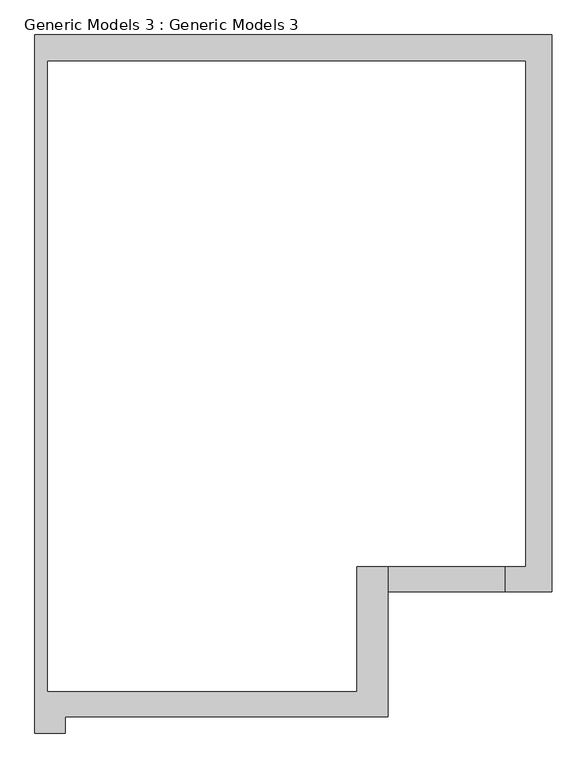
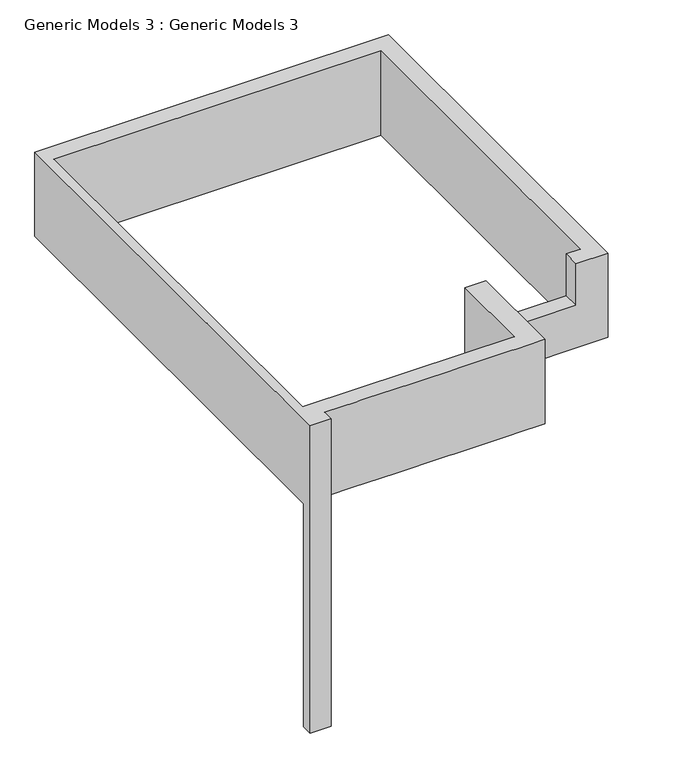
"""IFC4 building model written with IfcOpenShell, lengths in millimetres: proxy geometry, Generic Models 3 : Generic Models 3."""

from ifc_helpers import new_model, si_unit, origin, place, context, project, spatial, faceted_brep, source, transform, mapped, element, save


def generic_models_3_generic_models_3_92db7db1(model_context):
    return source(origin(), model_context, "Body", "Brep", [
        faceted_brep([(-12545.3628107, -11034.9642965, 8818.1896751), (-12545.3628107, -13359.0642965, 8818.1896751), (-18298.4628107, -13359.0642965, 8818.1896751), (-18298.4628107, -1646.3360225, 8818.1896751), (-9409.6215225, -1646.3360225, 8818.1896751), (-9409.6215225, -11034.9642965, 8818.1896751), (-9791.4069383, -11034.9642965, 8818.1896751), (-9791.4069383, -11497.6301294, 8818.1896751), (-8925.8628107, -11497.6301294, 8818.1896751), (-8925.8628107, -1167.0642965, 8818.1896751), (-18527.0628107, -1167.0642965, 8818.1896751), (-18527.0628107, -14121.0642965, 8818.1896751), (-17960.2455482, -14121.0642965, 8818.1896751), (-17960.2455482, -13816.2642965, 8818.1896751), (-17079.2628107, -13816.2642965, 8818.1896751), (-16980.0783065, -13816.2642965, 8818.1896751), (-16279.1628107, -13816.2642965, 8818.1896751), (-16187.9466003, -13816.2642965, 8818.1896751), (-15402.8628107, -13816.2642965, 8818.1896751), (-15312.895459, -13816.2642965, 8818.1896751), (-14567.4028515, -13816.2642965, 8818.1896751), (-14463.6220546, -13816.2642965, 8818.1896751), (-13726.4628107, -13816.2642965, 8818.1896751), (-13612.1628107, -13816.2642965, 8818.1896751), (-12879.2352221, -13816.2642965, 8818.1896751), (-12768.5357054, -13816.2642965, 8818.1896751), (-11973.8628107, -13816.2642965, 8818.1896751), (-11973.8628107, -11034.9642965, 8818.1896751), (-11973.8628107, -11497.6301294, 6400.8), (-11973.8628107, -13816.2642965, 6400.8), (-12768.5357054, -13816.2642965, 6400.8), (-12879.2352221, -13816.2642965, 6400.8), (-13612.1628107, -13816.2642965, 6400.8), (-13726.4628107, -13816.2642965, 6400.8), (-14463.6220546, -13816.2642965, 6400.8), (-14567.4028515, -13816.2642965, 6400.8), (-16187.9466003, -13816.2642965, 6400.8), (-16279.1628107, -13816.2642965, 6400.8), (-16980.0783065, -13816.2642965, 6400.8), (-17079.2628107, -13816.2642965, 6400.8), (-17960.2455482, -13816.2642965, 6400.8), (-18527.0628107, -13816.2642965, 6400.8), (-18527.0628107, -1167.0642965, 6400.8), (-8925.8628107, -1167.0642965, 6400.8), (-8925.8628107, -11497.6301294, 6400.8), (-12545.3628107, -13359.0642965, 6400.8), (-12545.3628107, -11034.9642965, 6400.8), (-9409.6215225, -11034.9642965, 6400.8), (-9409.6215225, -1646.3360225, 6400.8), (-18298.4628107, -1646.3360225, 6400.8), (-18298.4628107, -13359.0642965, 6400.8), (-11973.8628107, -11497.6301294, 7622.3726979), (-11973.8628107, -11034.9642965, 7622.3726979), (-18527.0628107, -13816.2642965, 0.0), (-18527.0628107, -14121.0642965, 0.0), (-9791.4069383, -11034.9642965, 7622.3726979), (-9791.4069383, -11497.6301294, 7622.3726979), (-17960.2455482, -14121.0642965, 0.0), (-17960.2455482, -13816.2642965, 0.0)], [[[0, 1, 2, 3, 4, 5, 6, 7, 8, 9, 10, 11, 12, 13, 14, 15, 16, 17, 18, 19, 20, 21, 22, 23, 24, 25, 26, 27]], [[28, 29, 30, 31, 32, 33, 34, 35, 36, 37, 38, 39, 40, 41, 42, 43, 44], [45, 46, 47, 48, 49, 50]], [[26, 29, 28, 51, 52, 27]], [[1, 45, 50, 2]], [[10, 42, 41, 53, 54, 11]], [[29, 26, 25, 24, 23, 22, 21, 20, 19, 18, 17, 16, 15, 14, 13, 40, 39, 38, 37, 36, 35, 34, 33, 32, 31, 30]], [[45, 1, 0, 46]], [[8, 44, 43, 9]], [[46, 0, 27, 52, 55, 6, 5, 47]], [[44, 8, 7, 56, 51, 28]], [[9, 43, 42, 10]], [[47, 5, 4, 48]], [[48, 4, 3, 49]], [[3, 2, 50, 49]], [[55, 56, 7, 6]], [[56, 55, 52, 51]], [[12, 11, 54, 57]], [[58, 53, 41, 40]], [[57, 54, 53, 58]], [[12, 57, 58, 40, 13]]]),
    ])


if __name__ == "__main__":
    model = new_model("IFC4")
    model_context = context("Model", 3, world=origin())
    ifc_project = project(units=[si_unit("LENGTHUNIT", "METRE", prefix="MILLI")], contexts=[model_context])
    site = spatial("IfcSite", under=ifc_project)
    building = spatial("IfcBuilding", under=site)
    placement = place(None, origin())
    generic_models_3_generic_models_3_shape = generic_models_3_generic_models_3_92db7db1(model_context)
    element("IfcBuildingElementProxy", 1, Name="Generic Models 3 : Generic Models 3", ObjectType="Generic Models 3 : Generic Models 3", at=placement, inside=building, context=model_context, shape_type="MappedRepresentation", body=[
        mapped(generic_models_3_generic_models_3_shape, transform((0.0, 0.0, 0.0), x_axis=(1.0, 0.0, 0.0), y_axis=(0.0, 1.0, 0.0), z_axis=(0.0, 0.0, 1.0))),
    ])
    save(model, "model.ifc")
